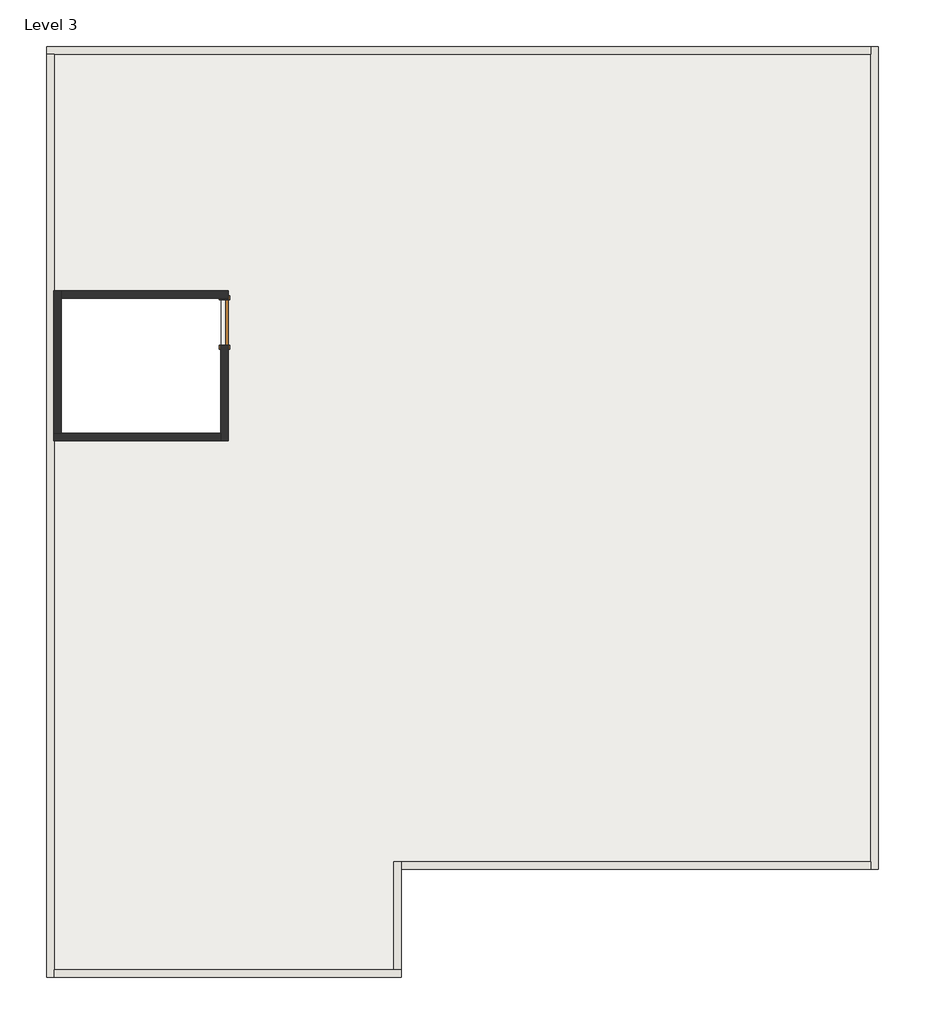
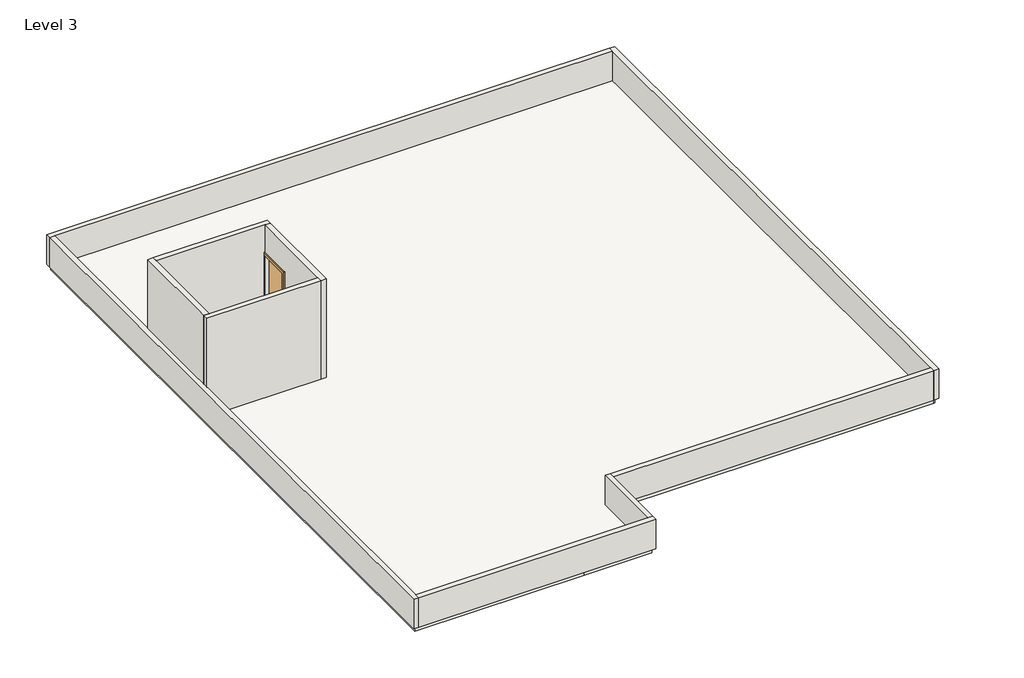
# One storey: 10 walls, 1 door, 1 slab.
"""IFC4 building model written with IfcOpenShell, lengths in millimetres."""

from ifc_helpers import new_model, si_unit, frame, origin, place, context, project, spatial, polyline, outline, extrude, faceted_brep, transform, mapped, element, save
from components import door_686f89d2

model = new_model("IFC4")

# Units and contexts
model_context = context("Model", 3, world=origin())
ifc_project = project(units=[si_unit("LENGTHUNIT", "METRE", prefix="MILLI")], contexts=[model_context])

# Site, building, storey
site = spatial("IfcSite", under=ifc_project)
building = spatial("IfcBuilding", under=site)
storey = spatial("IfcBuildingStorey", under=building, Name="Level 3", Elevation=6400.8)

# Door
placement = place(None, origin())
door_shape = door_686f89d2(model_context)
element("IfcDoor", 1, ObjectType="Single-Flush : 36\" x 84\"", at=placement, inside=storey, context=model_context, shape_type="MappedRepresentation", body=[
    mapped(door_shape, transform((-5812.0707895, 7223.9953048, 6400.8), x_axis=(0.0, 1.0, 0.0), y_axis=(-1.0, 0.0, 0.0), z_axis=(0.0, 0.0, 1.0))),
])

# Slab
element("IfcSlab", 2, ObjectType="6\"", at=placement, inside=storey, context=model_context, shape_type="SweptSolid", body=[
    extrude(outline(polyline([(-9292.4791271, -5780.8046952), (-9292.4791271, 12659.5144188), (7167.3292105, 12659.5144188), (7167.3292105, -3621.8046952), (7141.3208729, -3621.8046952), (-2358.2791271, -3621.8046952), (-2358.2791271, -5780.8046952), (-4339.4791271, -5780.8046952), (-9292.4791271, -5780.8046952)]), holes=[polyline([(-5888.2707895, 7706.5953048), (-9063.8791271, 7706.5953048), (-9063.8791271, 5014.1144188), (-5888.2707895, 5014.1144188), (-5888.2707895, 7706.5953048)])]), frame((0.0, 0.0, 6248.4), z_axis=(0.0, 0.0, 1.0), x_axis=(1.0, 0.0, 0.0)), (0.0, 0.0, 1.0), 152.4),
])

# Walls
element("IfcWall", 3, ObjectType="6\"", at=placement, inside=storey, context=model_context, shape_type="Brep", body=[
    faceted_brep([(-9368.0707895, 12583.3144188, 6400.8), (-9215.6707895, 12583.3144188, 6400.8), (7091.1292105, 12583.3144188, 6400.8), (7091.1292105, 12583.3144188, 7315.2), (-9215.6707895, 12583.3144188, 7315.2), (-9368.0707895, 12583.3144188, 7315.2), (-9368.0707895, 12735.7144188, 6400.8), (-9368.0707895, 12735.7144188, 7315.2), (7091.1292105, 12735.7144188, 7315.2), (7091.1292105, 12735.7144188, 6400.8)], [[[0, 1, 2, 3, 4, 5]], [[6, 7, 8, 9]], [[2, 1, 0, 6, 9]], [[5, 4, 3, 8, 7]], [[0, 5, 7, 6]], [[3, 2, 9, 8]]]),
])
element("IfcWall", 4, ObjectType="6\"", at=placement, inside=storey, context=model_context, shape_type="Brep", body=[
    faceted_brep([(-9215.6707895, -5857.0855812, 6400.8), (-9215.6707895, -5704.6855812, 6400.8), (-9215.6707895, 12583.3144188, 6400.8), (-9215.6707895, 12583.3144188, 7315.2), (-9215.6707895, -5704.6855812, 7315.2), (-9215.6707895, -5857.0855812, 7315.2), (-9368.0707895, -5857.0855812, 6400.8), (-9368.0707895, -5857.0855812, 7315.2), (-9368.0707895, 12583.3144188, 7315.2), (-9368.0707895, 12583.3144188, 6400.8)], [[[0, 1, 2, 3, 4, 5]], [[6, 7, 8, 9]], [[2, 1, 0, 6, 9]], [[5, 4, 3, 8, 7]], [[3, 2, 9, 8]], [[0, 5, 7, 6]]]),
])
element("IfcWall", 5, ObjectType="6\"", at=placement, inside=storey, context=model_context, shape_type="Brep", body=[
    faceted_brep([(7091.1292105, 12735.7144188, 6400.8), (7091.1292105, 12583.3144188, 6400.8), (7091.1292105, -3545.6046952, 6400.8), (7091.1292105, -3698.0046952, 6400.8), (7091.1292105, -3698.0046952, 7315.2), (7091.1292105, -3545.6046952, 7315.2), (7091.1292105, 12583.3144188, 7315.2), (7091.1292105, 12735.7144188, 7315.2), (7243.5292105, 12735.7144188, 6400.8), (7243.5292105, 12735.7144188, 7315.2), (7243.5292105, -3698.0046952, 7315.2), (7243.5292105, -3698.0046952, 6400.8)], [[[0, 1, 2, 3, 4, 5, 6, 7]], [[8, 9, 10, 11]], [[3, 2, 1, 0, 8, 11]], [[7, 6, 5, 4, 10, 9]], [[0, 7, 9, 8]], [[4, 3, 11, 10]]]),
])
element("IfcWall", 6, ObjectType="6\"", at=placement, inside=storey, context=model_context, shape_type="Brep", body=[
    faceted_brep([(-9215.6707895, -5857.0855812, 6400.8), (-2282.0791271, -5857.0855812, 6400.8), (-2282.0791271, -5857.0855812, 7315.2), (-9215.6707895, -5857.0855812, 7315.2), (-9215.6707895, -5704.6855812, 6400.8), (-9215.6707895, -5704.6855812, 7315.2), (-2434.4791271, -5704.6855812, 7315.2), (-2282.0791271, -5704.6855812, 7315.2), (-2282.0791271, -5704.6855812, 6400.8), (-2434.4791271, -5704.6855812, 6400.8)], [[[0, 1, 2, 3]], [[4, 5, 6, 7, 8, 9]], [[1, 0, 4, 9, 8]], [[3, 2, 7, 6, 5]], [[0, 3, 5, 4]], [[2, 1, 8, 7]]]),
])
element("IfcWall", 7, ObjectType="6\"", at=placement, inside=storey, context=model_context, shape_type="Brep", body=[
    faceted_brep([(-2282.0791271, -5704.6855812, 6400.8), (-2282.0791271, -3698.0046952, 6400.8), (-2282.0791271, -3545.6046952, 6400.8), (-2282.0791271, -3545.6046952, 7315.2), (-2282.0791271, -3698.0046952, 7315.2), (-2282.0791271, -5704.6855812, 7315.2), (-2434.4791271, -5704.6855812, 6400.8), (-2434.4791271, -5704.6855812, 7315.2), (-2434.4791271, -3545.6046952, 7315.2), (-2434.4791271, -3545.6046952, 6400.8)], [[[0, 1, 2, 3, 4, 5]], [[6, 7, 8, 9]], [[2, 1, 0, 6, 9]], [[5, 4, 3, 8, 7]], [[0, 5, 7, 6]], [[3, 2, 9, 8]]]),
])
element("IfcWall", 8, ObjectType="6\"", at=placement, inside=storey, context=model_context, shape_type="SweptSolid", body=[
    extrude(outline(polyline([(7091.1292105, -3698.0046952), (-2282.0791271, -3698.0046952), (-2282.0791271, -3545.6046952), (7091.1292105, -3545.6046952), (7091.1292105, -3698.0046952)])), frame((0.0, 0.0, 6400.8), z_axis=(0.0, 0.0, 1.0), x_axis=(1.0, 0.0, 0.0)), (0.0, 0.0, 1.0), 914.4),
])
element("IfcWall", 9, ObjectType="6\"", at=placement, inside=storey, context=model_context, shape_type="Brep", body=[
    faceted_brep([(-9070.2291271, 7706.5953048, 6400.8), (-5888.2707895, 7706.5953048, 6400.8), (-5735.8707895, 7706.5953048, 6400.8), (-5735.8707895, 7706.5953048, 9448.8), (-5888.2707895, 7706.5953048, 9448.8), (-9070.2291271, 7706.5953048, 9448.8), (-9070.2291271, 7858.9953048, 6400.8), (-9070.2291271, 7858.9953048, 9448.8), (-5735.8707895, 7858.9953048, 9448.8), (-5735.8707895, 7858.9953048, 6400.8)], [[[0, 1, 2, 3, 4, 5]], [[6, 7, 8, 9]], [[2, 1, 0, 6, 9]], [[5, 4, 3, 8, 7]], [[3, 2, 9, 8]], [[0, 5, 7, 6]]]),
])
element("IfcWall", 10, ObjectType="6\"", at=placement, inside=storey, context=model_context, shape_type="Brep", body=[
    faceted_brep([(-5888.2707895, 7706.5953048, 6400.8), (-5888.2707895, 7681.1953048, 6400.8), (-5888.2707895, 7681.1953048, 8534.4), (-5888.2707895, 6766.7953048, 8534.4), (-5888.2707895, 6766.7953048, 6400.8), (-5888.2707895, 5014.1953048, 6400.8), (-5888.2707895, 4861.7953048, 6400.8), (-5888.2707895, 4861.7953048, 9448.8), (-5888.2707895, 5014.1953048, 9448.8), (-5888.2707895, 7706.5953048, 9448.8), (-5735.8707895, 7681.1953048, 8534.4), (-5735.8707895, 7681.1953048, 6400.8), (-5735.8707895, 7706.5953048, 6400.8), (-5735.8707895, 7706.5953048, 9448.8), (-5735.8707895, 4861.7953048, 9448.8), (-5735.8707895, 4861.7953048, 6400.8), (-5735.8707895, 6766.7953048, 6400.8), (-5735.8707895, 6766.7953048, 8534.4)], [[[0, 1, 2, 3, 4, 5, 6, 7, 8, 9]], [[10, 11, 12, 13, 14, 15, 16, 17]], [[16, 15, 6, 5, 4]], [[12, 11, 1, 0]], [[9, 8, 7, 14, 13]], [[0, 9, 13, 12]], [[7, 6, 15, 14]], [[2, 1, 11, 10]], [[3, 2, 10, 17]], [[4, 3, 17, 16]]]),
])
element("IfcWall", 11, ObjectType="6\"", at=placement, inside=storey, context=model_context, shape_type="Brep", body=[
    faceted_brep([(-5888.2707895, 5014.1953048, 6400.8), (-9070.2291271, 5014.1953048, 6400.8), (-9222.6291271, 5014.1953048, 6400.8), (-9222.6291271, 5014.1953048, 9448.8), (-9070.2291271, 5014.1953048, 9448.8), (-5888.2707895, 5014.1953048, 9448.8), (-5888.2707895, 4861.7953048, 6400.8), (-5888.2707895, 4861.7953048, 9448.8), (-9222.6291271, 4861.7953048, 9448.8), (-9222.6291271, 4861.7953048, 6400.8)], [[[0, 1, 2, 3, 4, 5]], [[6, 7, 8, 9]], [[2, 1, 0, 6, 9]], [[5, 4, 3, 8, 7]], [[0, 5, 7, 6]], [[3, 2, 9, 8]]]),
])
element("IfcWall", 12, ObjectType="6\"", at=placement, inside=storey, context=model_context, shape_type="Brep", body=[
    faceted_brep([(-9070.2291271, 5014.1953048, 6400.8), (-9070.2291271, 7706.5953048, 6400.8), (-9070.2291271, 7858.9953048, 6400.8), (-9070.2291271, 7858.9953048, 9448.8), (-9070.2291271, 7706.5953048, 9448.8), (-9070.2291271, 5014.1953048, 9448.8), (-9222.6291271, 5014.1953048, 6400.8), (-9222.6291271, 5014.1953048, 9448.8), (-9222.6291271, 7858.9953048, 9448.8), (-9222.6291271, 7858.9953048, 6400.8)], [[[0, 1, 2, 3, 4, 5]], [[6, 7, 8, 9]], [[2, 1, 0, 6, 9]], [[5, 4, 3, 8, 7]], [[0, 5, 7, 6]], [[3, 2, 9, 8]]]),
])

save(model, "model.ifc")

# Revit data of these elements
# Type "Single-Flush : 36\" x 84\""
#   Type Mark = "1"
#   Construction Type Id = "MDOOR"
#   Assembly Code = "C1020"
#   Analytic Construction = "Metal"
#   Thickness = 0' - 2"
#   Heat Transfer Coefficient (U) = 0.651978 BTU/(h·ft²·°F)
#   Height = 7' - 0"
#   Trim Projection Ext = 0' - 1"
#   Trim Projection Int = 0' - 1"
#   Trim Width = 0' - 3"
#   Width = 3' - 0"
#   Define Thermal Properties by = 1
#   Door Material = Door - Panel
#   Frame Material = Door - Frame
#   Visual Light Transmittance = 0
#   Solar Heat Gain Coefficient = 0
#   Function = (empty or 0)
#   Wall Closure = (empty or 0)
# Type "6\""
#   Assembly Code = "B1010"
#   Function = 0
#   Layers, outside or top first: 0' - 6" "FLOOR" (function 1)
# Type "6\""
#   Assembly Code = "B2010"
#   Layers, outside or top first: 0' - 6" "INT WALL" (function 1)
# Element 1 (IfcDoor, "Single-Flush : 36\" x 84\"")
#   Phase Created = New Construction
#   Materials on its faces: "Door - Frame", "Door - Panel"
# Element 2 (IfcSlab, "6\"")
#   built-in parameter 1001955 = -1.5708 (stored number, unit not read)
#   Height Offset From Level = 0' - 0"
#   Phase Created = New Construction
#   Materials on its faces: "FLOOR"
# Elements 3, 4, 5, 6, 7, 8 (IfcWall, "6\"")
#   Top Offset = 0' - 0"
#   Base Offset = 0' - 0"
#   Unconnected Height = 3' - 0"
#   wall height = 3' - 0"
#   Phase Created = New Construction
#   Base Constraint = Level 3
#   Materials on its faces: "INT WALL"
# Elements 9, 10, 11, 12 (IfcWall, "6\"")
#   Top Offset = 0' - 0"
#   Base Offset = 0' - 0"
#   Unconnected Height = 10' - 0"
#   wall height = 10' - 0"
#   Phase Created = New Construction
#   Base Constraint = Level 3
#   Materials on its faces: "INT WALL"
# Materials
#   "Door - Panel": class "Wood", colour RGB 210 159 95, transparency 0
#   "Door - Frame": colour RGB 118 70 51, transparency 0
#   "FLOOR": class "Generic", colour RGB 140 134 116, transparency 0, Cost = 0
#   "INT WALL": class "Generic", colour RGB 164 133 98, transparency 0, Cost = 0
